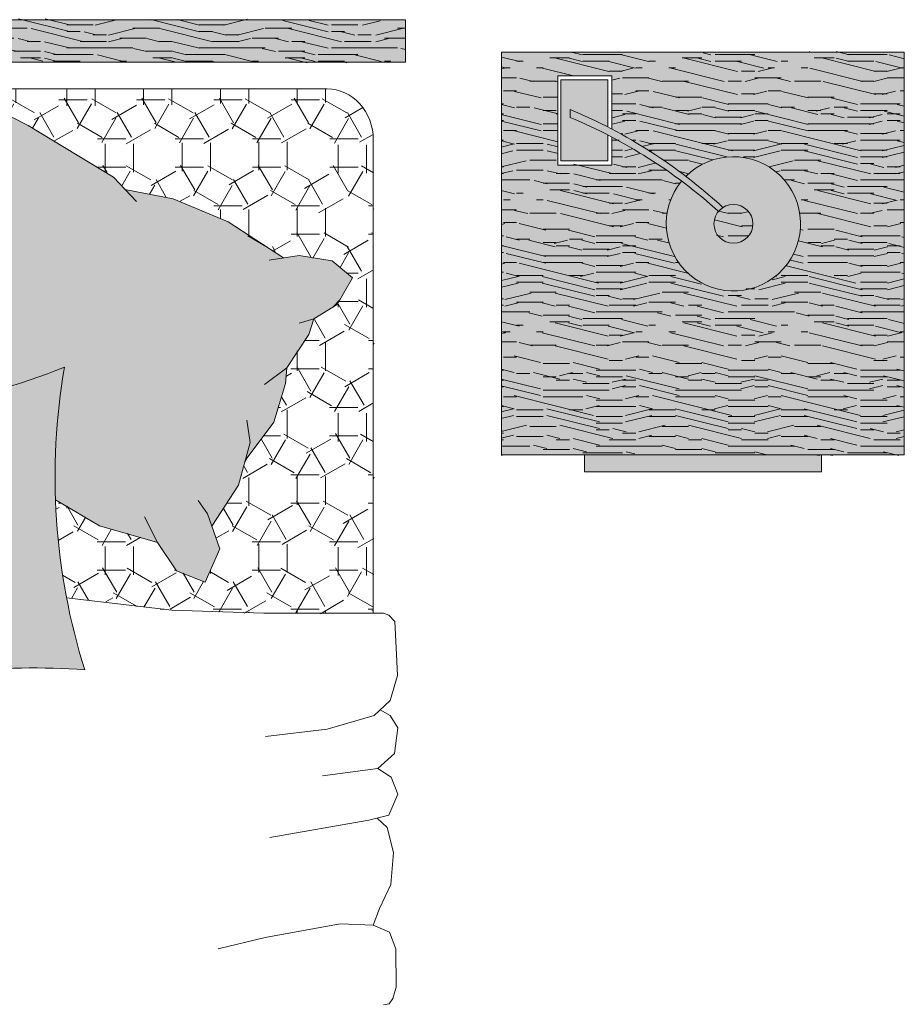
# Model space of a CAD drawing. Units: inches. Extents: x 1994 to 3075, y 3517 to 3950.
# Tile 46 of 58: x 1994.66748 to 1994.70433, y 3553.73529 to 3553.77632. Entities that reach past the tile are written whole.
import ezdxf

# ---------------------------------------------------------------- set-up
doc = ezdxf.new("R2010")
doc.units = ezdxf.units.IN
doc.layers.add('A-FURN-REFR', color=8, linetype='Continuous', lineweight=13)
doc.layers.add('A-FURN-REFR-PATT', color=8, linetype='Continuous', lineweight=13)
pattern_1 = [(0, (2000.713136654079, 3549.954056641144), (0, 0.005511811023622), [0.0011023622047244, -0.0016535433070866, 0.0005511811023622, -0.0022047244094488]), (0, (2000.716994921796, 3549.95419443642), (0, 0.005511811023622), [0.0011023622047244, -0.0044094488188976]), (0, (2000.716443740693, 3549.954470026972), (0, 0.005511811023622), [0.0005511811023622, -0.0049606299212598]), (0, (2000.71341224463, 3549.954607822247), (0, 0.005511811023622), [0.0002755905511811, -0.0038582677165354, 0.0002755905511811, -0.0011023622047244]), (0, (2000.715341378489, 3549.954883412798), (0, 0.005511811023622), [0.0011023622047244, -0.0016535433070866, 0.0002755905511811, -0.0024803149606299]), (0, (2000.713963425733, 3549.955021208074), (0, 0.005511811023622), [0.0008267716535433, -0.0046850393700787]), (0, (2000.715341378489, 3549.955159003349), (0, 0.005511811023622), [0.0016535433070866, -0.0038582677165354]), (0, (2000.713687835181, 3549.955296798625), (0, 0.005511811023622), [0.0011023622047244, -0.0044094488188976]), (0, (2000.715892559591, 3549.955434593901), (0, 0.005511811023622), [0.002755905511811, -0.002755905511811]), (0, (2000.714239016284, 3549.955710184451), (0, 0.005511811023622), [0.0005511811023622, -0.0016535433070866, 0.0011023622047244, -0.0022047244094488]), (0, (2000.718097284, 3549.955847979727), (0, 0.005511811023622), [0.0011023622047244, -0.0044094488188976]), (0, (2000.716994921796, 3549.955985775002), (0, 0.005511811023622), [0.0005511811023622, -0.0049606299212598]), (0, (2000.715892559591, 3549.956123570279), (0, 0.005511811023622), [0.0005511811023622, -0.0049606299212598]), (0, (2000.713136654079, 3549.956261365553), (0, 0.005511811023622), [0.0011023622047244, -0.0044094488188976]), (0, (2000.715892559591, 3549.956399160829), (0, 0.005511811023622), [0.0011023622047244, -0.0044094488188976]), (0, (2000.715892559591, 3549.95667475138), (0, 0.005511811023622), [0.0011023622047244, -0.0011023622047244, 0.0011023622047244, -0.0022047244094488]), (0, (2000.714790197386, 3549.956950341932), (0, 0.005511811023622), [0.0005511811023622, -0.002755905511811, 0.0011023622047244, -0.0011023622047244]), (0, (2000.715892559591, 3549.957088137207), (0, 0.005511811023622), [0.0016535433070866, -0.0038582677165354]), (0, (2000.715892559591, 3549.957363727759), (0, 0.005511811023622), [0.0011023622047244, -0.0044094488188976]), (0, (2000.713687835181, 3549.957501523034), (0, 0.005511811023622), [0.0016535433070866, -0.0022047244094488, 0.0005511811023622, -0.0011023622047244]), (0, (2000.713687835181, 3549.957777113585), (0, 0.005511811023622), [0.002755905511811, -0.002755905511811]), (0, (2000.716994921796, 3549.957914908861), (0, 0.005511811023622), [0.0005511811023622, -0.0049606299212598]), (0, (2000.715341378489, 3549.958052704136), (0, 0.005511811023622), [0.0011023622047244, -0.0044094488188976]), (0, (2000.714239016284, 3549.958190499412), (0, 0.005511811023622), [0.0005511811023622, -0.0022047244094488, 0.0005511811023622, -0.0022047244094488]), (0, (2000.713687835181, 3549.958328294688), (0, 0.005511811023622), [0.0005511811023622, -0.0016535433070866, 0.0011023622047244, -0.0022047244094488]), (0, (2000.714790197386, 3549.958466089964), (0, 0.005511811023622), [0.0005511811023622, -0.002755905511811, 0.0005511811023622, -0.0016535433070866]), (0, (2000.715892559591, 3549.958603885239), (0, 0.005511811023622), [0.0016535433070866, -0.0038582677165354]), (0, (2000.713687835181, 3549.95887947579), (0, 0.005511811023622), [0.0011023622047244, -0.0044094488188976]), (0, (2000.716443740693, 3549.959017271066), (0, 0.005511811023622), [0.0005511811023622, -0.0049606299212598]), (0, (2000.717546102898, 3549.959155066341), (0, 0.005511811023622), [0.0005511811023622, -0.0049606299212598]), (14.03624347, (2000.716994921796, 3549.954470026972), (0.0055118110234648, -2.016e-13), [0.0005677165354331, -0.0221580619543307]), (14.03624347, (2000.717546102898, 3549.955710184451), (0.0055118110234648, -2.016e-13), [0.0005677165354331, -0.0221580619543307]), (14.03624347, (2000.716994921796, 3549.959017271066), (0.0055118110234648, -2.016e-13), [0.0005677165354331, -0.0221580619543307]), (14.03624347, (2000.715341378489, 3549.956950341932), (0.0055118110234648, -2.016e-13), [0.0005677165354331, -0.0221580619543307]), (14.03624347, (2000.716443740693, 3549.957777113585), (0.0055118110234648, -2.016e-13), [0.0005677165354331, -0.0221580619543307]), (14.03624347, (2000.716994921796, 3549.957363727759), (0.0055118110234648, -2.016e-13), [0.0005677165354331, -0.0221580619543307]), (14.03624347, (2000.714239016284, 3549.958328294688), (0.0055118110234648, -2.016e-13), [0.0005677165354331, -0.0221580619543307]), (14.03624347, (2000.716443740693, 3549.958052704136), (0.0055118110234648, -2.016e-13), [0.0005677165354331, -0.0221580619543307]), (14.03624347, (2000.717546102898, 3549.955985775002), (0.0055118110234648, -2.016e-13), [0.0011354330708661, -0.0215903454188977]), (14.03624347, (2000.716994921796, 3549.956399160829), (0.0055118110234648, -2.016e-13), [0.0011354330708661, -0.0215903454188977]), (14.03624347, (2000.716994921796, 3549.95667475138), (0.0055118110234648, -2.016e-13), [0.0011354330708661, -0.0215903454188977]), (165.96375653, (2000.715341378489, 3549.954883412798), (-0.0055118110234648, -2.016e-13), [0.0005677165354331, -0.0011354330708661, 0.0005677165354331, -0.0204549123480315]), (165.96375653, (2000.714239016284, 3549.955710184451), (-0.0055118110234648, -2.016e-13), [0.0005677165354331, -0.0221580619543307]), (165.96375653, (2000.714239016284, 3549.958190499412), (-0.0055118110234648, -2.016e-13), [0.0011354330708661, -0.0215903454188977]), (194.03624347, (2000.716994921796, 3549.95419443642), (-0.0055118110234648, 2.016e-13), [0.0005677165354331, -0.0221580619543307]), (345.96375653, (2000.718097284, 3549.95419443642), (0.0055118110234648, 2.016e-13), [0.0005677165354331, -0.0221580619543307]), (345.96375653, (2000.716443740693, 3549.956123570279), (0.0055118110234648, 2.016e-13), [0.0005677165354331, -0.0221580619543307]), (345.96375653, (2000.717546102898, 3549.957088137207), (0.0055118110234648, 2.016e-13), [0.0005677165354331, -0.0221580619543307]), (345.96375653, (2000.715341378489, 3549.957501523034), (0.0055118110234648, 2.016e-13), [0.0005677165354331, -0.0221580619543307]), (345.96375653, (2000.714790197386, 3549.958190499412), (0.0055118110234648, 2.016e-13), [0.0005677165354331, -0.0221580619543307]), (345.96375653, (2000.715341378489, 3549.958466089964), (0.0055118110234648, 2.016e-13), [0.0005677165354331, -0.0221580619543307]), (345.96375653, (2000.715341378489, 3549.957501523034), (0.0055118110234648, 2.016e-13), [0.0005677165354331, -0.0221580619543307]), (345.96375653, (2000.716994921796, 3549.958328294688), (0.0055118110234648, 2.016e-13), [0.0022708661417323, -0.0204549123480315]), (345.96375653, (2000.713687835181, 3549.954607822247), (0.0055118110234648, 2.016e-13), [0.0022708661417323, -0.0204549123480315]), (345.96375653, (2000.714239016284, 3549.955021208074), (0.0055118110234648, 2.016e-13), [0.0022708661417323, -0.0204549123480315]), (345.96375653, (2000.714790197386, 3549.955296798625), (0.0055118110234648, 2.016e-13), [0.0005677165354331, -0.0011354330708661, 0.0011354330708661, -0.0198871958125984]), (345.96375653, (2000.714790197386, 3549.955710184451), (0.0055118110234648, 2.016e-13), [0.0011354330708661, -0.0011354330708661, 0.0011354330708661, -0.0193194792771654]), (345.96375653, (2000.714239016284, 3549.956261365553), (0.0055118110234648, 2.016e-13), [0.0022708661417323, -0.0204549123480315]), (345.96375653, (2000.713687835181, 3549.95667475138), (0.0055118110234648, 2.016e-13), [0.0022708661417323, -0.0204549123480315]), (345.96375653, (2000.713687835181, 3549.956950341932), (0.0055118110234648, 2.016e-13), [0.0022708661417323, -0.0204549123480315]), (345.96375653, (2000.717546102898, 3549.958603885239), (0.0055118110234648, 2.016e-13), [0.0005677165354331, -0.0221580619543307]), (345.9637675300001, (2000.718097284, 3549.959155066341), (0.0055118110234647, 1.0583933e-09), [0.0011354330708661, -0.0215903454188977]), (345.9637675300001, (2000.714790197386, 3549.95887947579), (0.0055118110234647, 1.0583933e-09), [0.0011354330708661, -0.0215903454188977]), (345.96375753, (2000.714239016284, 3549.954056641144), (0.0055118110234648, 9.64008e-11), [0.0022708661417323, -0.0204549123480315]), (345.96375753, (2000.717546102898, 3549.957914908861), (0.0055118110234648, 9.64008e-11), [0.0017031496062992, -0.0210226288834646]), (345.96375753, (2000.718097284, 3549.957501523034), (0.0055118110234648, 9.64008e-11), [0.0034062992125984, -0.0193194792771654])]

msp = doc.modelspace()

# ---------------------------------------------------------------- hatches: boundary and pattern name
at = {"layer": 'A-FURN-REFR-PATT'}
for points in [[(1994.683554943529, 3553.776316211922), (1994.629017487434, 3553.776316211922), (1994.629017487434, 3553.774548566426), (1994.683554943529, 3553.774548566426)], [(1994.691973859139, 3553.773803717286), (1994.690026984246, 3553.773803717286), (1994.690026984246, 3553.770436718028), (1994.691973859139, 3553.770436718028), (1994.691973859139, 3553.771515132102, 0.0198106445216623), (1994.690411703692, 3553.772242175532), (1994.690411703692, 3553.772573101428, -0.0198106445216993), (1994.691973859139, 3553.771846057998), (1994.691973859139, 3553.77185293988)]]:
    msp.add_hatch(color=256, dxfattribs=at).paths.add_polyline_path(points)
h = msp.add_hatch(dxfattribs=at)
h.set_pattern_fill('LEGNO1', color=256, scale=0.005511811023622, style=0, pattern_type=2)
h.set_pattern_definition(pattern_1)
h.paths.add_polyline_path([(1994.683554943529, 3553.776316211922), (1994.629017487434, 3553.776316211922), (1994.629017487434, 3553.774548566426), (1994.683554943529, 3553.774548566426)])
h = msp.add_hatch(color=256, dxfattribs=at)
h.paths.add_polyline_path([(1994.704329684038, 3553.774969762488), (1994.687546825394, 3553.774969762488), (1994.687546825394, 3553.758186903844), (1994.704329684038, 3553.758186903844)])
h.paths.add_polyline_path([(1994.695053205861, 3553.769589737948, 0.0395152736214826), (1994.692150847766, 3553.771423035513), (1994.692150847766, 3553.770259509415), (1994.689894243114, 3553.770259509415), (1994.689894243114, 3553.7739809259), (1994.692150847766, 3553.7739809259), (1994.692150847766, 3553.771753961409, -0.042086183498597), (1994.695231327647, 3553.769785957469, -42.19598506439468)], flags=16)
h.paths.add_polyline_path([(1994.696401056411, 3553.767809896967, -1), (1994.698020989977, 3553.767809896967, -1)], flags=0)
h = msp.add_hatch(dxfattribs=at)
h.set_pattern_fill('LEGNO1', color=256, scale=0.005511811023622, style=0, pattern_type=2)
h.set_pattern_definition(pattern_1)
h.paths.add_polyline_path([(1994.704329684038, 3553.774969762488), (1994.687546825394, 3553.774969762488), (1994.687546825394, 3553.758186903844), (1994.704329684038, 3553.758186903844)])
h.paths.add_polyline_path([(1994.689894243114, 3553.770259509415), (1994.689894243114, 3553.7739809259), (1994.692150847766, 3553.7739809259), (1994.692150847766, 3553.771753961409, -0.042086183498597), (1994.695231327647, 3553.769785957469, -42.19598506432865), (1994.695053205861, 3553.769589737948, 0.0395152736214861), (1994.692150847766, 3553.771423035513), (1994.692150847766, 3553.770259509415)], flags=16)
h.paths.add_polyline_path([(1994.696401056411, 3553.767809896967, -1), (1994.698020989977, 3553.767809896967, -1)], flags=0)
h = msp.add_hatch(color=256, dxfattribs=at)
h.set_gradient(color1=(238, 215, 180), color2=(243, 226, 201), one_color=1, tint=0.8700000047683715)
edge = h.paths.add_edge_path()
edge.add_line((1994.676159070622, 3553.767890272889), (1994.673866270238, 3553.768856171096))
edge.add_line((1994.673866270238, 3553.768856171096), (1994.671861384366, 3553.769242244476))
edge.add_line((1994.671861384366, 3553.769242244476), (1994.671386706816, 3553.769751038746))
edge.add_line((1994.671386706816, 3553.769751038746), (1994.667830227734, 3553.771901929654))
edge.add_line((1994.667830227734, 3553.771901929654), (1994.665734215684, 3553.77297958654))
edge.add_line((1994.665734215684, 3553.77297958654), (1994.665026572095, 3553.773822225779))
edge.add_line((1994.665026572095, 3553.773822225779), (1994.663883992918, 3553.774548566426))
edge.add_line((1994.663883992918, 3553.774548566426), (1994.658782089951, 3553.774548566426))
edge.add_line((1994.658782089951, 3553.774548566426), (1994.658800201509, 3553.774325920301))
edge.add_line((1994.658800201509, 3553.774325920301), (1994.657843589582, 3553.77321545307))
edge.add_line((1994.657843589582, 3553.77321545307), (1994.657422550984, 3553.771734332495))
edge.add_line((1994.657422550984, 3553.771734332495), (1994.656565089816, 3553.770144665209))
edge.add_line((1994.656565089816, 3553.770144665209), (1994.65570185959, 3553.769069712963))
edge.add_line((1994.65570185959, 3553.769069712963), (1994.655112675836, 3553.767735644958))
edge.add_line((1994.655112675836, 3553.767735644959), (1994.65530000938, 3553.767274460835))
edge.add_line((1994.65530000938, 3553.767274460835), (1994.655602453494, 3553.765603625222))
edge.add_line((1994.655602453494, 3553.765603625222), (1994.655292057156, 3553.763678547347))
edge.add_line((1994.655292057156, 3553.763678547347), (1994.655292057156, 3553.763480373162))
edge.add_line((1994.655292057156, 3553.763480373162), (1994.655293013242, 3553.76347580391))
edge.add_line((1994.655293013242, 3553.76347580391), (1994.655860621967, 3553.763271787719))
edge.add_line((1994.655860621967, 3553.763271787719), (1994.656620872249, 3553.7635037195))
edge.add_line((1994.656620872249, 3553.7635037195), (1994.657838944906, 3553.762473458848))
edge.add_line((1994.657838944906, 3553.762473458848), (1994.660448145662, 3553.761168419415))
edge.add_line((1994.660448145662, 3553.761168419415), (1994.661752586042, 3553.760238020281))
edge.add_ellipse((1994.661382372394, 3553.784798673296), major_axis=(-6.65e-14, 0.0245640191959876), ratio=0.9104034055871746, start_angle=180.863579370377, end_angle=184.4498598488241)
edge.add_ellipse((1994.661382372394, 3553.784798673296), major_axis=(-6.65e-14, 0.0245640191959876), ratio=0.9104034055871746, start_angle=184.4498598488241, end_angle=194.3650168968225)
edge.add_ellipse((1994.661382372394, 3553.784798673296), major_axis=(-6.65e-14, 0.0245640191959876), ratio=0.9104034055871746, start_angle=194.3650168968225, end_angle=199.1150547931432)
edge.add_ellipse((1994.691382311155, 3553.757287383518), major_axis=(1.05e-14, 0.0246376990644585), ratio=0.9104034055889432, start_angle=78.32633054579424, end_angle=85.22710521724885)
edge.add_ellipse((1994.691382311155, 3553.757287383518), major_axis=(1.05e-14, 0.0246376990644585), ratio=0.9104034055889432, start_angle=85.22710521724885, end_angle=92.51657122573107)
edge.add_line((1994.668970000248, 3553.756302346309), (1994.670799258103, 3553.755226460611))
edge.add_line((1994.670799258103, 3553.755226460611), (1994.673214003473, 3553.754536678136))
edge.add_line((1994.673214003473, 3553.754536678136), (1994.674008849961, 3553.753345682028))
edge.add_line((1994.674008849961, 3553.753345682028), (1994.675201941324, 3553.752880490442))
edge.add_line((1994.675201941324, 3553.752880490442), (1994.67581166639, 3553.754261069415))
edge.add_line((1994.67581166639, 3553.754261069415), (1994.675476739891, 3553.755213492086))
edge.add_line((1994.675476739891, 3553.755213492086), (1994.676594694229, 3553.756913681281))
edge.add_line((1994.676594694229, 3553.756913681282), (1994.676870413768, 3553.757942127319))
edge.add_line((1994.676870413768, 3553.757942127319), (1994.678065726595, 3553.75954078439))
edge.add_line((1994.678065726595, 3553.75954078439), (1994.678547737755, 3553.761159962988))
edge.add_line((1994.678547737755, 3553.761159962988), (1994.678602941398, 3553.761812736369))
edge.add_line((1994.678602941398, 3553.761812736369), (1994.679525220981, 3553.763197317897))
edge.add_line((1994.679525220981, 3553.763197317897), (1994.679736701813, 3553.763852092397))
edge.add_line((1994.679736701814, 3553.763852092397), (1994.680539099516, 3553.764348808849))
edge.add_line((1994.680539099516, 3553.764348808849), (1994.680822868901, 3553.764660505163))
edge.add_line((1994.680822868901, 3553.764660505162), (1994.681343139427, 3553.7655543089))
edge.add_line((1994.681343139427, 3553.7655543089), (1994.680491166369, 3553.766264103519))
edge.add_line((1994.680491166368, 3553.766264103519), (1994.679113235034, 3553.766486692973))
edge.add_line((1994.679113235034, 3553.766486692973), (1994.678460266424, 3553.766388571271))
edge.add_line((1994.678460266424, 3553.766388571271), (1994.676159070622, 3553.767890272889))
h = msp.add_hatch(dxfattribs=at)
h.set_pattern_fill('ESA_QT1', color=256, scale=0.0011811023622047, style=0, pattern_type=2)
h.set_pattern_definition([(0, (2000.713136654079, 3549.955670026971), (0.0016133858267717, 0.0027944881889764), [0.0011811023622047, -0.0020457874015748]), (0, (2000.713136654079, 3549.956851129334), (0.0016133858267717, 0.0027944881889764), [0.0011811023622047, -0.0020457874015748]), (60, (2000.714750748567, 3549.954056641144), (-0.0016134048488433, 0.0027944772065782), [0.0011811023622047, -0.0020457874015748]), (60, (2000.71372720526, 3549.954647192326), (-0.0016134048488433, 0.0027944772065782), [0.0011811023622047, -0.0020457874015748]), (119.9999999999999, (2000.715931142268, 3549.954056641144), (-0.0032267906756149, -1.09823982e-08), [0.0011811023622047, -0.0020457874015748]), (119.9999999999999, (2000.716954095024, 3549.954647192326), (-0.0032267906756149, -1.09823982e-08), [0.0011811023622047, -0.0020457874015748]), (90, (2000.713136654079, 3549.955670026971), (-0.0016133858267717, 0.0027944881889764), [0.0011811023622047, -0.0044079921259843]), (90, (2000.714317756441, 3549.955670026971), (-0.0016133858267717, 0.0027944881889764), [0.0011811023622047, -0.0044079921259843]), (30, (2000.715931142268, 3549.954056641144), (0.0016134048488433, 0.0027944772065782), [0.0011811023622047, -0.0044079921259843]), (150, (2000.714750039906, 3549.954056641144), (-0.0032267906756149, 1.09823982e-08), [0.0011811023622047, -0.0044079921259843]), (30, (2000.715340591087, 3549.95507947579), (0.0016134048488433, 0.0027944772065782), [0.0011811023622047, -0.0044079921259843]), (150, (2000.715340591087, 3549.95507947579), (-0.0032267906756149, 1.09823982e-08), [0.0011811023622047, -0.0044079921259843])])
edge = h.paths.add_edge_path()
edge.add_ellipse((1994.640876267803, 3553.752583994587), major_axis=(5.1e-14, 0.0199705920159029), ratio=0.9104034055885663, start_angle=279.2384781746984, end_angle=295.7125839497674)
edge.add_ellipse((1994.661382372394, 3553.784798673296), major_axis=(-6.65e-14, 0.0245640191959876), ratio=0.9104034055871746, start_angle=170.9484486625179, end_angle=180.863579370377)
edge.add_line((1994.661752586042, 3553.760238020281), (1994.660448145662, 3553.761168419415))
edge.add_line((1994.660448145662, 3553.761168419415), (1994.657838944906, 3553.762473458848))
edge.add_line((1994.657838944906, 3553.762473458848), (1994.656620872249, 3553.7635037195))
edge.add_line((1994.656620872249, 3553.7635037195), (1994.655860621967, 3553.763271787719))
edge.add_line((1994.655860621967, 3553.763271787719), (1994.655293013242, 3553.76347580391))
edge.add_line((1994.655293013242, 3553.76347580391), (1994.655492642102, 3553.762521752315))
edge.add_line((1994.655492642102, 3553.762521752315), (1994.655292057156, 3553.760583980486))
edge.add_line((1994.655292057156, 3553.760583980486), (1994.655292057156, 3553.760424196786))
edge.add_line((1994.655292057156, 3553.760424196786), (1994.655993894027, 3553.759788080461))
edge.add_line((1994.655993894027, 3553.759788080461), (1994.656078542309, 3553.758256449834))
edge.add_line((1994.656078542309, 3553.758256449834), (1994.65483102117, 3553.758019537339))
edge.add_line((1994.65483102117, 3553.758019537339), (1994.653606721018, 3553.758629674708))
edge.add_line((1994.653606721018, 3553.758629674708), (1994.651194153521, 3553.757930758213))
edge.add_line((1994.651194153521, 3553.757930758214), (1994.647696839888, 3553.757851284215))
edge.add_line((1994.647696839888, 3553.757851284214), (1994.645838514283, 3553.758007709834))
edge.add_line((1994.645838514283, 3553.758007709834), (1994.644835983502, 3553.757660521972))
edge.add_line((1994.644835983502, 3553.757660521972), (1994.641770029086, 3553.757379220126))
edge.add_line((1994.641770029086, 3553.757379220126), (1994.639520236034, 3553.757536658586))
edge.add_line((1994.639520236035, 3553.757536658586), (1994.636663612057, 3553.757269314918))
edge.add_line((1994.636663612057, 3553.757269314918), (1994.635142148634, 3553.757511478539))
edge.add_line((1994.635142148634, 3553.757511478539), (1994.6345829999, 3553.756899988171))
edge.add_line((1994.6345829999, 3553.756899988171), (1994.633060603732, 3553.756567883332))
edge.add_line((1994.633060603732, 3553.756567883332), (1994.631935706918, 3553.756646602719))
edge.add_line((1994.631935706918, 3553.756646602719), (1994.631946230123, 3553.757723396824))
edge.add_line((1994.631946230123, 3553.757723396824), (1994.632292941058, 3553.759053199603))
edge.add_line((1994.632292941058, 3553.759053199604), (1994.631941882006, 3553.760336474997))
edge.add_line((1994.631941882006, 3553.760336474997), (1994.631857233723, 3553.761868105623))
edge.add_line((1994.631857233724, 3553.761868105623), (1994.632129935231, 3553.763269837439))
edge.add_line((1994.632129935231, 3553.763269837439), (1994.632167911274, 3553.765117099948))
edge.add_line((1994.632167911274, 3553.765117099948), (1994.631873931996, 3553.766634772358))
edge.add_line((1994.631873931997, 3553.766634772358), (1994.632212178095, 3553.768117738339))
edge.add_line((1994.632212178095, 3553.768117738339), (1994.631520698886, 3553.769224586838))
edge.add_line((1994.631520698886, 3553.769224586838), (1994.631256346504, 3553.770206188564))
edge.add_line((1994.631256346504, 3553.770206188563), (1994.631719391006, 3553.770698246991))
edge.add_line((1994.631719391006, 3553.770698246991), (1994.632687804151, 3553.770916548533))
edge.add_line((1994.632687804151, 3553.770916548533), (1994.633747155817, 3553.770756594945))
edge.add_line((1994.633747155817, 3553.770756594945), (1994.634990443991, 3553.77107008883))
edge.add_line((1994.634990443991, 3553.77107008883), (1994.637863997621, 3553.771031106442))
edge.add_line((1994.637863997621, 3553.771031106442), (1994.638856831888, 3553.770677652785))
edge.add_line((1994.638856831888, 3553.770677652785), (1994.641164677522, 3553.770866877247))
edge.add_line((1994.641164677522, 3553.770866877247), (1994.645224440128, 3553.770906991414))
edge.add_line((1994.645224440128, 3553.770906991414), (1994.645865234264, 3553.770719090863))
edge.add_line((1994.645865234264, 3553.770719090863), (1994.647785025882, 3553.771462050497))
edge.add_line((1994.647785025882, 3553.771462050497), (1994.650214523032, 3553.771854640936))
edge.add_line((1994.650214523032, 3553.771854640936), (1994.652890445746, 3553.771784733682))
edge.add_line((1994.652890445747, 3553.771784733682), (1994.653415799595, 3553.772221829723))
edge.add_line((1994.653415799595, 3553.772221829723), (1994.654716167523, 3553.772769720975))
edge.add_line((1994.654716167523, 3553.772769720975), (1994.655775519189, 3553.772609767387))
edge.add_line((1994.655775519189, 3553.772609767387), (1994.65570791623, 3553.771298575913))
edge.add_line((1994.65570791623, 3553.771298575913), (1994.655134945204, 3553.770261141011))
edge.add_line((1994.655134945204, 3553.770261141011), (1994.655242813935, 3553.769576559863))
edge.add_line((1994.655242813935, 3553.769576559863), (1994.655056819059, 3553.76787315508))
edge.add_line((1994.655056819059, 3553.76787315508), (1994.655112675836, 3553.767735644959))
edge.add_line((1994.655112675836, 3553.767735644959), (1994.65570185959, 3553.769069712964))
edge.add_line((1994.65570185959, 3553.769069712963), (1994.656565089816, 3553.770144665209))
edge.add_line((1994.656565089816, 3553.770144665209), (1994.657422550984, 3553.771734332495))
edge.add_line((1994.657422550984, 3553.771734332495), (1994.657843589582, 3553.77321545307))
edge.add_line((1994.657843589582, 3553.77321545307), (1994.65802844368, 3553.77343003791))
edge.add_line((1994.65802844368, 3553.77343003791), (1994.632243770886, 3553.77343003791))
edge.add_ellipse((1994.632243770886, 3553.771319321668), major_axis=(1.39e-14, 0.0021107162422937), ratio=0.9104034055886554, start_angle=3.727201e-10, end_angle=90.00000000038261)
edge.add_line((1994.630322167631, 3553.771319321668), (1994.630322167631, 3553.749440774068))
edge.add_line((1994.630322167631, 3553.749440774068), (1994.637708571751, 3553.750433433404))
edge.add_line((1994.637708571751, 3553.750433433405), (1994.645848690548, 3553.752087865434))
edge.add_line((1994.645848690548, 3553.752087865434), (1994.649253851983, 3553.752270169246))
edge.add_line((1994.649253851983, 3553.752270169246), (1994.654398272776, 3553.75242317871))
edge.add_line((1994.654398272776, 3553.75242317871), (1994.656592872189, 3553.752620614647))
edge.add_ellipse((1994.639937157511, 3553.760628246485), major_axis=(3.09e-14, 0.0199705920159139), ratio=0.9104034055882502, start_angle=244.3229699956078, end_angle=253.1594339628131)
edge.add_ellipse((1994.674343922271, 3553.771436729311), major_axis=(9.73e-14, 0.0245640191959803), ratio=0.9104034055882507, start_angle=133.6720839547031, end_angle=139.6806386089699)
edge.add_line((1994.659095375291, 3553.753468572294), (1994.658861443608, 3553.755509353953))
edge = h.paths.add_edge_path()
edge.add_ellipse((1994.680283852266, 3553.771319321668), major_axis=(7.5e-15, 0.0021107162422937), ratio=0.9104034055891856, start_angle=270.0000000002102, end_angle=360.0000000002004)
edge.add_line((1994.680283852266, 3553.77343003791), (1994.665355929212, 3553.77343003791))
edge.add_line((1994.665355929212, 3553.77343003791), (1994.665734215684, 3553.77297958654))
edge.add_line((1994.665734215684, 3553.77297958654), (1994.667830227734, 3553.771901929654))
edge.add_line((1994.667830227734, 3553.771901929654), (1994.671386706816, 3553.769751038746))
edge.add_line((1994.671386706816, 3553.769751038746), (1994.671861384366, 3553.769242244476))
edge.add_line((1994.671861384366, 3553.769242244476), (1994.673866270238, 3553.768856171096))
edge.add_line((1994.673866270238, 3553.768856171096), (1994.676159070622, 3553.767890272889))
edge.add_line((1994.676159070622, 3553.767890272889), (1994.678460266424, 3553.766388571271))
edge.add_line((1994.678460266424, 3553.766388571271), (1994.679113235034, 3553.766486692973))
edge.add_line((1994.679113235034, 3553.766486692973), (1994.680491166368, 3553.766264103519))
edge.add_line((1994.680491166368, 3553.766264103519), (1994.681343139427, 3553.7655543089))
edge.add_line((1994.681343139427, 3553.7655543089), (1994.680699082158, 3553.764447844539))
edge.add_line((1994.680699082158, 3553.764447844539), (1994.679736701814, 3553.763852092397))
edge.add_line((1994.679736701814, 3553.763852092397), (1994.679525220982, 3553.763197317897))
edge.add_line((1994.679525220981, 3553.763197317897), (1994.678602941398, 3553.761812736369))
edge.add_line((1994.678602941398, 3553.761812736369), (1994.678547737755, 3553.761159962988))
edge.add_line((1994.678547737755, 3553.761159962988), (1994.678065726595, 3553.75954078439))
edge.add_line((1994.678065726595, 3553.75954078439), (1994.676936092021, 3553.758029967927))
edge.add_line((1994.676936092021, 3553.758029967927), (1994.676847654697, 3553.757857234982))
edge.add_line((1994.676847654697, 3553.757857234982), (1994.676594694229, 3553.756913681281))
edge.add_line((1994.676594694229, 3553.756913681282), (1994.675476739891, 3553.755213492087))
edge.add_line((1994.675476739891, 3553.755213492086), (1994.67581166639, 3553.754261069415))
edge.add_line((1994.67581166639, 3553.754261069415), (1994.675201941324, 3553.752880490442))
edge.add_line((1994.675201941324, 3553.752880490442), (1994.674008849961, 3553.753345682028))
edge.add_line((1994.674008849961, 3553.753345682028), (1994.673214003473, 3553.754536678136))
edge.add_line((1994.673214003473, 3553.754536678136), (1994.670799258103, 3553.755226460611))
edge.add_line((1994.670799258103, 3553.755226460611), (1994.668970000248, 3553.756302346308))
edge.add_ellipse((1994.691382311155, 3553.757287383518), major_axis=(1.05e-14, 0.0246376990644585), ratio=0.9104034055889432, start_angle=92.51657122573107, end_angle=102.9728254987549)
edge.add_line((1994.669429675006, 3553.752230183665), (1994.673814418644, 3553.751710497517))
edge.add_line((1994.673814418644, 3553.751710497517), (1994.677652873975, 3553.7515865923))
edge.add_line((1994.677652873975, 3553.7515865923), (1994.682205455522, 3553.7515865923))
edge.add_line((1994.682205455522, 3553.7515865923), (1994.682205455522, 3553.755102098136))
edge.add_line((1994.682205455522, 3553.755102098136), (1994.682205455522, 3553.771319321668))
h = msp.add_hatch(color=256, dxfattribs=at)
h.dxf.hatch_style = 1
h.set_gradient(color1=(167, 169, 175), one_color=1, tint=1)
h.paths.add_polyline_path([(1994.690411703692, 3553.772242175532), (1994.690411703692, 3553.772573101428, -0.0875286051314429), (1994.696772375269, 3553.768490803852, 0.0763380806476787), (1994.696588272154, 3553.768327803648, 0.0846435149619904)])
h = msp.add_hatch(color=256, dxfattribs=at)
h.dxf.hatch_style = 1
h.set_gradient(color1=(37, 53, 157), color2=(142, 207, 230), tint=1, name='SPHERICAL')
h.paths.add_polyline_path([(1994.697211023195, 3553.76861986375, 0.1440580758931676), (1994.696772375269, 3553.768490803852, 0.0231477939795123), (1994.695231327647, 3553.769785957469, -42.19598506439846), (1994.695053205861, 3553.769589737948, -0.0228504078660832), (1994.696588272154, 3553.768327803648, 0.6355278128427492), (1994.697211023195, 3553.766999930184, 1)])
h = msp.add_hatch(color=256, dxfattribs=at)
h.dxf.hatch_style = 1
h.set_gradient(color1=(37, 40, 142), tint=1, name='INVSPHERICAL')
h.paths.add_polyline_path([(1994.697211023195, 3553.766999930184, -1), (1994.697211023195, 3553.76861986375, -1)])
h = msp.add_hatch(color=256, dxfattribs=at)
h.set_gradient(color1=(223, 184, 155), color2=(248, 239, 232), one_color=1, tint=0.9399999976158142, name='SPHERICAL')
edge = h.paths.add_edge_path()
edge.add_ellipse((1994.691382311155, 3553.757287383518), major_axis=(1.05e-14, 0.0246376990644585), ratio=0.9104034055889432, start_angle=92.51657122573113, end_angle=102.97282549875501, ccw=False)
edge.add_ellipse((1994.691382311155, 3553.757287383518), major_axis=(1.05e-14, 0.0246376990644585), ratio=0.9104034055889432, start_angle=78.32633054579418, end_angle=92.51657122573113, ccw=False)
edge.add_ellipse((1994.661382372394, 3553.784798673296), major_axis=(-6.65e-14, 0.0245640191959876), ratio=0.9104034055871746, start_angle=180.8635793703771, end_angle=199.1150547931432, ccw=False)
edge.add_ellipse((1994.661382372394, 3553.784798673296), major_axis=(-6.65e-14, 0.0245640191959876), ratio=0.9104034055871746, start_angle=170.948448662518, end_angle=180.8635793703771, ccw=False)
edge.add_ellipse((1994.640876267803, 3553.752583994587), major_axis=(5.1e-14, 0.0199705920159029), ratio=0.9104034055885663, start_angle=279.2384781746984, end_angle=295.71258394976746, ccw=False)
edge.add_line((1994.658861443608, 3553.755509353953), (1994.659095375291, 3553.753468572294))
edge.add_ellipse((1994.674343922271, 3553.771436729311), major_axis=(9.73e-14, 0.0245640191959803), ratio=0.9104034055882507, start_angle=139.6806386089699, end_angle=157.0382139804205)
edge.add_ellipse((1994.667940210471, 3553.708562887745), major_axis=(1.025e-13, 0.0407397684618791), ratio=0.9104034055980798, start_angle=356.86033449210555, end_angle=364.2705504231131, ccw=False)
edge.add_line((1994.670170840053, 3553.749228911329), (1994.67018195311, 3553.749241118068))
edge.add_ellipse((1994.691382311155, 3553.757287383518), major_axis=(1.05e-14, 0.0246376990644585), ratio=0.9104034055889432, start_angle=102.97282549875501, end_angle=110.78347723807451, ccw=False)
h = msp.add_hatch(color=256, dxfattribs=at)
h.set_gradient(color1=(158, 155, 166), rotation=89.99999999999996, one_color=1, tint=1)
h.paths.add_polyline_path([(1994.70087598743, 3553.758186903844), (1994.691000522003, 3553.758186903844), (1994.691000522003, 3553.757480977518), (1994.70087598743, 3553.757480977518)])

# ---------------------------------------------------------------- linework, layer by layer
at = {"layer": 'A-FURN-REFR'}
for p, q in [((1994.683554943529, 3553.776316211922), (1994.629017487434, 3553.776316211922)), ((1994.683554943529, 3553.774548566426), (1994.683554943529, 3553.776316211922)), ((1994.687546825394, 3553.774969762488), (1994.687546825394, 3553.758186903844)), ((1994.704329684038, 3553.774969762488), (1994.687546825394, 3553.774969762488)), ((1994.704329684038, 3553.758186903844), (1994.704329684038, 3553.774969762488)), ((1994.629017487434, 3553.774548566426), (1994.683554943529, 3553.774548566426)), ((1994.665355929212, 3553.77343003791), (1994.680283852266, 3553.77343003791)), ((1994.665734215684, 3553.77297958654), (1994.667830227734, 3553.771901929654)), ((1994.690411703692, 3553.772573101428), (1994.690411703692, 3553.772242175532)), ((1994.667830227734, 3553.771901929654), (1994.671386706816, 3553.769751038746)), ((1994.682205455522, 3553.755102098136), (1994.682205455522, 3553.771319321668)), ((1994.671386706816, 3553.769751038746), (1994.672335907567, 3553.768733615649)), ((1994.671861384366, 3553.769242244476), (1994.673866270238, 3553.768856171096)), ((1994.673866270238, 3553.768856171096), (1994.676159070622, 3553.767890272889)), ((1994.676159070622, 3553.767890272889), (1994.678460266424, 3553.766388571271)), ((1994.679113235034, 3553.766486692973), (1994.677864940167, 3553.766299111494)), ((1994.680491166368, 3553.766264103519), (1994.679113235034, 3553.766486692973)), ((1994.681343139427, 3553.7655543089), (1994.680491166368, 3553.766264103519)), ((1994.680699082158, 3553.764447844539), (1994.681343139427, 3553.7655543089)), ((1994.679736701814, 3553.763852092397), (1994.680699082158, 3553.764447844539)), ((1994.680539099516, 3553.764348808849), (1994.680822868901, 3553.764660505162)), ((1994.679113515844, 3553.763672515712), (1994.679736701814, 3553.763852092397)), ((1994.679525220981, 3553.763197317897), (1994.679736701814, 3553.763852092397)), ((1994.678602941398, 3553.761812736369), (1994.679525220981, 3553.763197317897)), ((1994.677672969829, 3553.761114441773), (1994.678602941398, 3553.761812736369)), ((1994.678547737755, 3553.761159962988), (1994.678602941398, 3553.761812736369)), ((1994.678065726595, 3553.75954078439), (1994.678547737755, 3553.761159962988)), ((1994.676870413768, 3553.757942127319), (1994.678065726595, 3553.75954078439)), ((1994.677074782603, 3553.758704432087), (1994.676939376713, 3553.759629318643)), ((1994.676594694229, 3553.756913681282), (1994.677074782603, 3553.758704432087)), ((1994.676847654697, 3553.757857234982), (1994.676936092021, 3553.758029967927)), ((1994.687546825394, 3553.758186903844), (1994.704329684038, 3553.758186903844)), ((1994.675476739891, 3553.755213492086), (1994.676594694229, 3553.756913681282)), ((1994.668970000248, 3553.756302346309), (1994.670799258103, 3553.755226460611)), ((1994.675295041712, 3553.755730182956), (1994.674913822786, 3553.756274409626)), ((1994.67581166639, 3553.754261069415), (1994.675295041712, 3553.755730182956)), ((1994.672670738438, 3553.755593619042), (1994.673214003473, 3553.754536678136)), ((1994.670799258103, 3553.755226460611), (1994.673214003473, 3553.754536678136)), ((1994.682205455522, 3553.755102098136), (1994.682205455522, 3553.7515865923)), ((1994.673214003473, 3553.754536678136), (1994.674008849961, 3553.753345682028)), ((1994.675201941324, 3553.752880490442), (1994.67581166639, 3553.754261069415)), ((1994.674008849961, 3553.753345682028), (1994.675201941324, 3553.752880490442)), ((1994.669429675006, 3553.752230183665), (1994.673814418644, 3553.751710497517)), ((1994.673814418644, 3553.751710497517), (1994.677652873975, 3553.7515865923)), ((1994.677652873975, 3553.7515865923), (1994.682205455522, 3553.7515865923)), ((1994.682205455522, 3553.7515865923), (1994.682630764051, 3553.7515865923)), ((1994.682630764051, 3553.7515865923), (1994.682852272648, 3553.751505273051)), ((1994.682852272648, 3553.751505273051), (1994.683101432613, 3553.751231815691)), ((1994.683101432613, 3553.751231815691), (1994.683172620965, 3553.749858017436)), ((1994.683172620965, 3553.749858017436), (1994.683219253014, 3553.748992543795)), ((1994.670170840053, 3553.749228911329), (1994.67018195311, 3553.749241118068)), ((1994.683219253014, 3553.748992543795), (1994.682912123693, 3553.747950660672)), ((1994.682912123693, 3553.747950660672), (1994.682250206595, 3553.747323213443)), ((1994.682496171722, 3553.747556369737), (1994.682905130062, 3553.747323213443)), ((1994.682250206595, 3553.747323213443), (1994.680285437616, 3553.746758450657)), ((1994.682905130062, 3553.747323213443), (1994.683232591085, 3553.746809793054)), ((1994.680285437616, 3553.746758450657), (1994.677712526535, 3553.746450398067)), ((1994.683232591085, 3553.746809793054), (1994.683092249834, 3553.745731608986)), ((1994.683092249834, 3553.745731608986), (1994.682390547845, 3553.745115503805)), ((1994.680098316423, 3553.744807451214), (1994.682390547845, 3553.745115503805)), ((1994.682390547845, 3553.745115503805), (1994.682951910005, 3553.744756108818)), ((1994.682951910005, 3553.744756108818), (1994.683232591085, 3553.744037319738)), ((1994.683232591085, 3553.744037319738), (1994.682858350119, 3553.743164504362)), ((1994.682858350119, 3553.743164504362), (1994.682016305459, 3553.742959135671)), ((1994.682373674903, 3553.743046295531), (1994.682782266641, 3553.742655596482)), ((1994.682016305459, 3553.742959135671), (1994.677899647728, 3553.74224034659)), ((1994.682782266641, 3553.742655596482), (1994.68304701293, 3553.741609572409)), ((1994.68304701293, 3553.741609572409), (1994.682941114415, 3553.740272984951)), ((1994.682941114415, 3553.740272984951), (1994.682464572516, 3553.739285072483)), ((1994.682464572516, 3553.739285072483), (1994.682199827648, 3553.738587723398)), ((1994.680823152631, 3553.738645835897), (1994.677699160634, 3553.738064710915)), ((1994.682199827648, 3553.738587723398), (1994.680823152631, 3553.738645835897)), ((1994.682888165158, 3553.738297160908), (1994.682199827648, 3553.738587723398)), ((1994.68314674348, 3553.737594421543), (1994.682888165158, 3553.738297160908)), ((1994.677699160634, 3553.738064710915), (1994.675740046623, 3553.737599810931)), ((1994.68316189335, 3553.735994289664), (1994.68314674348, 3553.737594421543)), ((1994.683019516646, 3553.735532016407), (1994.68316189335, 3553.735994289664)), ((1994.682630764051, 3553.735263176962), (1994.68287120758, 3553.735310646031)), ((1994.68287120758, 3553.735310646031), (1994.683019516646, 3553.735532016407))]:
    msp.add_line(p, q, dxfattribs=at)
for points in [[(1994.692150847766, 3553.771753961409), (1994.692150847766, 3553.7739809259), (1994.689894243114, 3553.7739809259), (1994.689894243114, 3553.770259509415), (1994.692150847766, 3553.770259509415), (1994.692150847766, 3553.771423035513)], [(1994.691973859139, 3553.771846057998), (1994.691973859139, 3553.773803717286), (1994.690026984246, 3553.773803717286), (1994.690026984246, 3553.770436718028), (1994.691973859139, 3553.770436718028), (1994.691973859139, 3553.771515132102)], [(1994.691973859139, 3553.771846057998), (1994.691973859139, 3553.77185293988)], [(1994.692150847766, 3553.771753961409), (1994.692150847766, 3553.771757928811)]]:
    msp.add_lwpolyline(points, dxfattribs=at)
msp.add_lwpolyline([(1994.691000522003, 3553.757480977518), (1994.691000522003, 3553.758186903844), (1994.70087598743, 3553.758186903844), (1994.70087598743, 3553.757480977518)], close=True, dxfattribs=at)
msp.add_circle((1994.697211023195, 3553.767809896967), 0.0008099667829119, dxfattribs=at)
for centre, radius, start, end in [((1994.682021473379, 3553.752503729669), 0.0217526009365345, 47.30299182645985, 67.31207620217475), ((1994.682021473379, 3553.752172803773), 0.0217526009365345, 47.95934126430827, 67.31207620217475), ((1994.697211023195, 3553.767809896967), 0.002797143107239, 140.4830303783151, 135.0526505436044)]:
    msp.add_arc(centre, radius, start, end, dxfattribs=at)
at = {"layer": 'A-FURN-REFR', "extrusion": (0, 0, -1)}
for centre, major_axis, ratio, start_param, end_param in [((1994.680283852266, 3553.771319321668), (7.5e-15, 0.0021107162422937), 0.9104034055891856, -3.8418e-12, 1.570796326791555), ((1994.661382372394, 3553.784798673296), (-6.65e-14, 0.0245640191959876), 0.9104034055871746, 2.777848732022604, 3.314823705227802), ((1994.691382311155, 3553.757287383518), (1.05e-14, 0.0246376990644585), 0.9104034055889432, 4.379134586166689, 4.898315717548383), ((1994.667940210471, 3553.708562887745), (1.025e-13, 0.0407397684618791), 0.9104034055980798, -0.0818392287954246, 0.0605905375575699)]:
    msp.add_ellipse(centre, major_axis=major_axis, ratio=ratio, start_param=start_param, end_param=end_param, dxfattribs=at)

doc.saveas('drawing.dxf')
